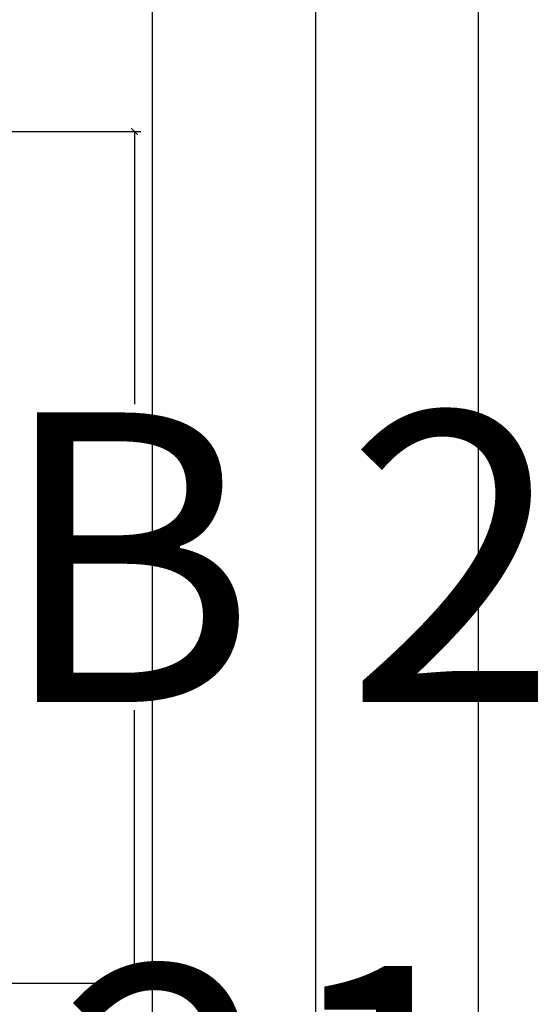
# Model space of a CAD drawing. Units: inches. Extents: x -48 to 50072, y 0 to 21068.
# Tile 37 of 75: x 541 to 555, y 251 to 279. Entities that reach past the tile are written whole.
import ezdxf

# ---------------------------------------------------------------- set-up
doc = ezdxf.new("R2010")
doc.units = ezdxf.units.IN
doc.header["$MEASUREMENT"] = 0
doc.linetypes.add('ACAD_ISO02W100', pattern=[15, 12, -3])
for name, color, linetype, lineweight in [('A-ANNO-DIMS', 2, 'Continuous', 18), ('C-PROP', 7, 'Continuous', 25), ('C-PROP-REF', 32, 'ACAD_ISO02W100', 13)]:
    doc.layers.add(name, color=color, linetype=linetype, lineweight=lineweight)
doc.styles.get("Standard").update_dxf_attribs({"font": 'arial.ttf'})
doc.dimstyles.get("Standard").update_dxf_attribs({"dimtxt": 8, "dimasz": 0.18, "dimexe": 0.18, "dimexo": 0.0625, "dimgap": 0.09, "dimtad": 0, "dimtih": 1, "dimtoh": 1, "dimdec": 1, "dimzin": 0, "dimdsep": 46, "dimlunit": 4, "dimtxsty": 'Standard', "dimblk": 'ARCHTICK', "dimcen": 0.09, "dimadec": 0, "dimazin": 0, "dimtfac": 1, "dimtdec": 1, "dimtofl": 0, "dimtmove": 0, "dimatfit": 3, "dimldrblk": 'ARCHTICK', "dimfxl": 1, "dimtolj": 1, "dimtzin": 0, "dimarcsym": 0})

# ---------------------------------------------------------------- blocks, each defined once
blk = doc.blocks.new('_ArchTick')
at = {"color": 0, "linetype": 'ByBlock', "const_width": 0.15}
blk.add_lwpolyline([(-0.5, -0.5), (0.5, 0.5)], dxfattribs=at)
blk = doc.blocks.new('*D54')
at = {"layer": 'A-ANNO-DIMS', "color": 0, "lineweight": -2, "transparency": 16777216}
for p, q in [((540.551, 275.597), (544.198, 275.597)), ((544.018, 275.597), (544.018, 268.06)), ((544.018, 252.07), (544.018, 259.607)), ((540.551, 252.07), (544.198, 252.07))]:
    blk.add_line(p, q, dxfattribs=at)
at = {"layer": 'Defpoints', "color": 0, "transparency": 16777216}
for p in [(540.489, 275.597), (544.018, 275.597), (540.489, 252.07)]:
    blk.add_point(p, dxfattribs=at)
at = {"layer": 'A-ANNO-DIMS', "color": 0, "lineweight": -2, "transparency": 16777216, "xscale": 0.18, "yscale": 0.18, "zscale": 0.18}
for p, rotation in [((544.018, 275.597), 90), ((544.018, 252.07), 270)]:
    blk.add_blockref('_ArchTick', p, dxfattribs=dict(at, rotation=rotation))
at = {"layer": 'A-ANNO-DIMS', "color": 0, "transparency": 16777216, "insert": (544.018, 263.834), "char_height": 8, "attachment_point": 5}
blk.add_mtext('\\A1;SHRUB B 24 TYP.', dxfattribs=at)
blk = doc.blocks.new('*D55')
at = {"layer": 'A-ANNO-DIMS', "color": 0, "lineweight": -2, "transparency": 16777216}
for p, q in [((519.098, 252.008), (519.098, 248.361)), ((540.489, 252.008), (540.489, 248.361)), ((519.098, 248.541), (540.489, 248.541)), ((540.489, 248.541), (540.669, 248.541))]:
    blk.add_line(p, q, dxfattribs=at)
at = {"layer": 'Defpoints', "color": 0, "transparency": 16777216}
for p in [(519.098, 252.07), (540.489, 252.07), (540.489, 248.541)]:
    blk.add_point(p, dxfattribs=at)
at = {"layer": 'A-ANNO-DIMS', "color": 0, "lineweight": -2, "transparency": 16777216, "xscale": 0.18, "yscale": 0.18, "zscale": 0.18, "rotation": 180}
blk.add_blockref('_ArchTick', (519.098, 248.541), dxfattribs=at)
at = {"layer": 'A-ANNO-DIMS', "color": 0, "lineweight": -2, "transparency": 16777216, "xscale": 0.18, "yscale": 0.18, "zscale": 0.18}
blk.add_blockref('_ArchTick', (540.489, 248.541), dxfattribs=at)
at = {"layer": 'A-ANNO-DIMS', "color": 0, "transparency": 16777216, "insert": (560.298, 248.541), "char_height": 8, "attachment_point": 5}
blk.add_mtext('\\A1;21 TYP.', dxfattribs=at)
blk = doc.blocks.new('*D115')
at = {"layer": 'A-ANNO-DIMS', "color": 0, "lineweight": -2, "transparency": 16777216}
for p, q in [((549.08, 451.075), (601.647, 451.075)), ((601.467, 451.075), (601.467, 336.752)), ((601.467, 214.075), (601.467, 328.397)), ((553.58, 214.075), (601.647, 214.075))]:
    blk.add_line(p, q, dxfattribs=at)
at = {"layer": 'Defpoints', "color": 0, "transparency": 16777216}
for p in [(549.017, 451.075), (601.467, 451.075), (553.517, 214.075)]:
    blk.add_point(p, dxfattribs=at)
at = {"layer": 'A-ANNO-DIMS', "color": 0, "lineweight": -2, "transparency": 16777216, "xscale": 0.18, "yscale": 0.18, "zscale": 0.18}
for p, rotation in [((601.467, 451.075), 90), ((601.467, 214.075), 270)]:
    blk.add_blockref('_ArchTick', p, dxfattribs=dict(at, rotation=rotation))
at = {"layer": 'A-ANNO-DIMS', "color": 0, "transparency": 16777216, "insert": (601.467, 332.575), "char_height": 8, "attachment_point": 5}
blk.add_mtext('\\A1;237', dxfattribs=at)
blk = doc.blocks.new('*D119')
at = {"layer": 'A-ANNO-DIMS', "color": 0, "lineweight": -2, "transparency": 16777216}
for p, q in [((463.517, 451.012), (463.517, 165.945)), ((549.017, 451.012), (549.017, 165.945)), ((463.517, 166.125), (495.752, 166.125)), ((549.017, 166.125), (516.783, 166.125))]:
    blk.add_line(p, q, dxfattribs=at)
at = {"layer": 'Defpoints', "color": 0, "transparency": 16777216}
for p in [(463.517, 451.075), (549.017, 451.075), (549.017, 166.125)]:
    blk.add_point(p, dxfattribs=at)
at = {"layer": 'A-ANNO-DIMS', "color": 0, "lineweight": -2, "transparency": 16777216, "xscale": 0.18, "yscale": 0.18, "zscale": 0.18, "rotation": 180}
blk.add_blockref('_ArchTick', (463.517, 166.125), dxfattribs=at)
at = {"layer": 'A-ANNO-DIMS', "color": 0, "lineweight": -2, "transparency": 16777216, "xscale": 0.18, "yscale": 0.18, "zscale": 0.18}
blk.add_blockref('_ArchTick', (549.017, 166.125), dxfattribs=at)
at = {"layer": 'A-ANNO-DIMS', "color": 0, "transparency": 16777216, "insert": (506.267, 166.125), "char_height": 8, "attachment_point": 5}
blk.add_mtext('\\A1;85.5', dxfattribs=at)

msp = doc.modelspace()

# ---------------------------------------------------------------- linework, layer by layer
at = {"layer": 'C-PROP'}
for p, q in [((553.517, 214.075), (553.517, 1170.775)), ((544.517, 223.075), (544.517, 488.775))]:
    msp.add_line(p, q, dxfattribs=at)
at = {"layer": 'C-PROP-REF'}
msp.add_line((549.017, 214.075), (549.017, 1166.275), dxfattribs=at)

# ---------------------------------------------------------------- dimensions: what is measured, and where the dimension line sits
at = {"layer": 'A-ANNO-DIMS'}
dim = msp.add_linear_dim(base=(549.017, 166.125), p1=(463.517, 451.075), p2=(549.017, 451.075), dimstyle='Standard', override={"dimdec": 1, "dimlfac": 1, "dimrnd": 0, "dimzin": 0, "dimdsep": 46, "dimlunit": 2}, dxfattribs=at)
dim.commit()
dim.dimension.update_dxf_attribs({"geometry": '*D119', "text_midpoint": (506.267, 166.125)})
dim = msp.add_linear_dim(base=(601.467, 451.075), p1=(553.517, 214.075), p2=(549.017, 451.075), angle=90, dimstyle='Standard', override={"dimdec": 0, "dimlfac": 1, "dimrnd": 0, "dimzin": 0, "dimdsep": 46, "dimlunit": 2}, dxfattribs=at)
dim.commit()
dim.dimension.update_dxf_attribs({"geometry": '*D115', "text_midpoint": (601.467, 332.575)})
dim = msp.add_linear_dim(base=(544.018, 275.597), p1=(540.489, 252.07), p2=(540.489, 275.597), angle=90, text='SHRUB B <> TYP.', dimstyle='Standard', override={"dimdec": 0, "dimlfac": 1, "dimrnd": 0, "dimzin": 0, "dimdsep": 46, "dimlunit": 2}, dxfattribs=at)
dim.commit()
dim.dimension.update_dxf_attribs({"geometry": '*D54', "text_midpoint": (544.018, 263.834)})
dim = msp.add_linear_dim(base=(540.489, 248.541), p1=(519.098, 252.07), p2=(540.489, 252.07), text='<> TYP.', dimstyle='Standard', override={"dimdec": 0, "dimlfac": 1, "dimrnd": 0, "dimzin": 0, "dimdsep": 46, "dimlunit": 2}, dxfattribs=at)
dim.commit()
dim.dimension.update_dxf_attribs({"geometry": '*D55', "text_midpoint": (560.298, 248.541)})

doc.saveas('drawing.dxf')
